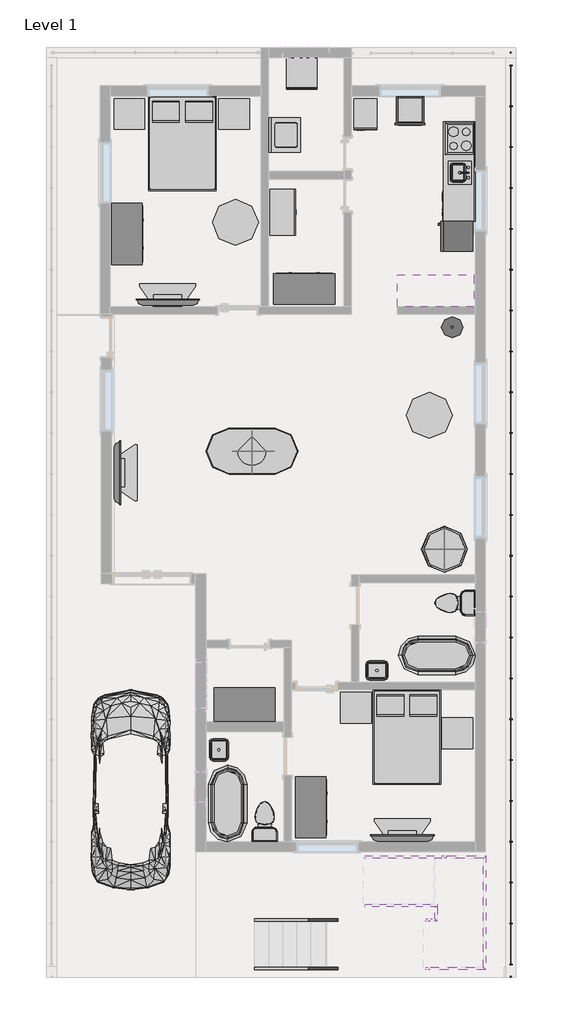
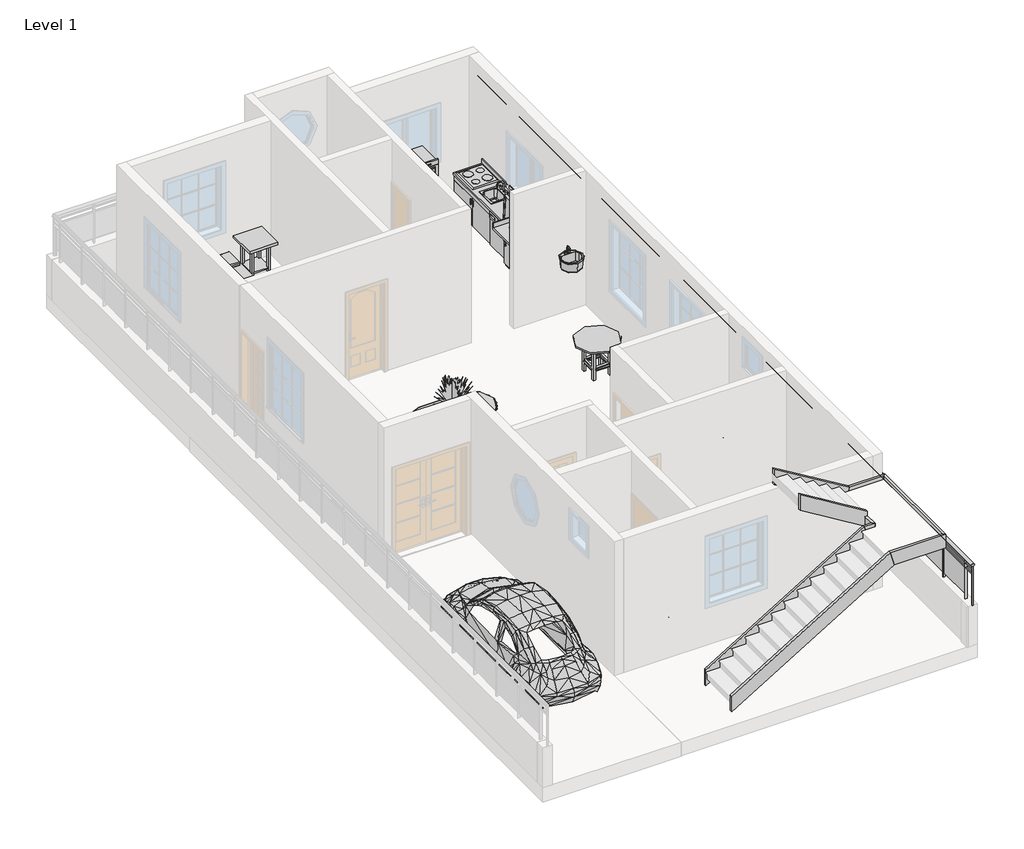
# One storey, part 3 of 3: 23 furniture elements, 9 members, 9 proxies, 8 flow terminals, 2 geographic elements, 1 railing.
"""IFC4 building model written with IfcOpenShell, lengths in millimetres."""

from ifc_helpers import new_model, si_unit, point, frame, origin, place, context, project, spatial, polyline, ellipse_curve, trimmed, outline, extrude, faceted_brep, transform, mapped, element, save
from ifc_brep_helpers import plane_surface, extruded_surface, advanced_brep
from components import proxy_7e1014cc, proxy_a6faaae8, proxy_45b28599, kitchenette_medium_kitchenette_medium_844211aa, proxy_8b8c2dc4, rpc_beetle_rpc_beetle_3ce7ba48, proxy_c523a7b7, proxy_718fa39f, flow_terminal_871c2e40, flow_terminal_d49f872f, flow_terminal_62a433f7, toilet_domestic_3d_toilet_domestic_3d_f7549cf7, toilet_domestic_3d_toilet_domestic_3d_183bbd19, flow_terminal_b374fae2, furniture_c8abb964, furniture_c6510c7c, furniture_6430aa70, furniture_2babcf72, furniture_9fa109b2, furniture_80f2079a, furniture_e1dba61b, furniture_fdf74506, tv_stand_tv_stand_6ce107e5, furniture_2c34a4f9, furniture_905aceb5, furniture_4bee3317, furniture_5bc9ed15, furniture_c80d6d9c, rpc_plant_tropical_agave_1_5_93a2a214, rpc_plant_tropical_dagger_2_80c14bd7

model = new_model("IFC4")

# Units and contexts
model_context = context("Model", 3, world=origin())
ifc_project = project(units=[si_unit("LENGTHUNIT", "METRE", prefix="MILLI")], contexts=[model_context])

# Site, building, storey
site = spatial("IfcSite", under=ifc_project)
building = spatial("IfcBuilding", under=site)
storey = spatial("IfcBuildingStorey", under=building, Name="Level 1", Elevation=0.0)

# Proxies
placement = place(None, origin())
proxy_shape = proxy_7e1014cc(model_context)
element("IfcBuildingElementProxy", 1, Name="18\" x 24\" x 34 1/2\"", ObjectType="18\" x 24\" x 34 1/2\"", at=placement, inside=storey, context=model_context, shape_type="MappedRepresentation", body=[
    mapped(proxy_shape, transform((-1733.5258635, 13886.7655534, 0.0), x_axis=(1.0, 0.0, 0.0), y_axis=(0.0, 1.0, 0.0), z_axis=(0.0, 0.0, 1.0))),
])
proxy_2_shape = proxy_a6faaae8(model_context)
element("IfcBuildingElementProxy", 2, Name="Cook Top-4 Unit2 : 22\" x 20\"", ObjectType="Cook Top-4 Unit2 : 22\" x 20\"", at=placement, inside=storey, context=model_context, shape_type="MappedRepresentation", body=[
    mapped(proxy_2_shape, transform((452.191605, 13657.9151182, 0.0), x_axis=(0.0, -1.0000000000000004, 0.0), y_axis=(1.0000000000000004, 0.0, 0.0), z_axis=(0.0, 0.0, 1.0))),
])
proxy_3_shape = proxy_45b28599(model_context)
element("IfcBuildingElementProxy", 3, Name="Dishwasher : 24\" x 24\" x 34\"", ObjectType="Dishwasher : 24\" x 24\" x 34\"", at=placement, inside=storey, context=model_context, shape_type="MappedRepresentation", body=[
    mapped(proxy_3_shape, transform((-3079.7258635, 14699.5655534, 0.0), x_axis=(1.0, 0.0, 0.0), y_axis=(0.0, 1.0, 0.0), z_axis=(0.0, 0.0, 1.0))),
])
element("IfcBuildingElementProxy", 4, Name="Dishwasher : 24\" x 24\" x 34\"", ObjectType="Dishwasher : 24\" x 24\" x 34\"", at=placement, inside=storey, context=model_context, shape_type="MappedRepresentation", body=[
    mapped(proxy_3_shape, transform((160.3420402, 12706.7325867, 0.0), x_axis=(0.0, -1.0000000000000004, 0.0), y_axis=(1.0000000000000004, 0.0, 0.0), z_axis=(0.0, 0.0, 1.0))),
])
kitchenette_medium_kitchenette_medium_shape = kitchenette_medium_kitchenette_medium_844211aa(model_context)
element("IfcBuildingElementProxy", 5, Name="Kitchenette - Medium : Kitchenette - Medium", ObjectType="Kitchenette - Medium : Kitchenette - Medium", at=placement, inside=storey, context=model_context, shape_type="MappedRepresentation", body=[
    mapped(kitchenette_medium_kitchenette_medium_shape, transform((756.991605, 13333.7528231, 0.0), x_axis=(0.0, -1.0000000000000004, 0.0), y_axis=(1.0000000000000004, 0.0, 0.0), z_axis=(0.0, 0.0, 1.0))),
])
proxy_4_shape = proxy_8b8c2dc4(model_context)
element("IfcBuildingElementProxy", 6, Name="Oven Double-Built-in : 21 1/2\" x 39 1/4\" x 21\"", ObjectType="Oven Double-Built-in : 21 1/2\" x 39 1/4\" x 21\"", at=placement, inside=storey, context=model_context, shape_type="MappedRepresentation", body=[
    mapped(proxy_4_shape, transform((-503.2334677, 14088.3492592, 0.0), x_axis=(1.0, 0.0, 0.0), y_axis=(0.0, 1.0, 0.0), z_axis=(0.0, 0.0, 1.0))),
])
rpc_beetle_rpc_beetle_shape = rpc_beetle_rpc_beetle_3ce7ba48(model_context)
element("IfcBuildingElementProxy", 7, Name="RPC Beetle : RPC Beetle", ObjectType="RPC Beetle : RPC Beetle", at=placement, inside=storey, context=model_context, shape_type="MappedRepresentation", body=[
    mapped(rpc_beetle_rpc_beetle_shape, transform((-6101.008395, -527.9848818, 0.0), x_axis=(1.0, 0.0, 0.0), y_axis=(0.0, 1.0, 0.0), z_axis=(0.0, 0.0, 1.0))),
])
proxy_5_shape = proxy_c523a7b7(model_context)
element("IfcBuildingElementProxy", 8, Name="Refrigerator : 24\" x 25\" LH", ObjectType="Refrigerator : 24\" x 25\" LH", at=placement, inside=storey, context=model_context, shape_type="MappedRepresentation", body=[
    mapped(proxy_5_shape, transform((406.5426335, 11721.1651182, 0.0), x_axis=(0.0, -1.0000000000000004, 0.0), y_axis=(1.0000000000000004, 0.0, 0.0), z_axis=(0.0, 0.0, 1.0))),
])
proxy_6_shape = proxy_718fa39f(model_context)
element("IfcBuildingElementProxy", 9, Name="Washer : 27\" x 25\" x 35\"", ObjectType="Washer : 27\" x 25\" x 35\"", at=placement, inside=storey, context=model_context, shape_type="MappedRepresentation", body=[
    mapped(proxy_6_shape, transform((-2761.1588302, 13313.6976497, 0.0), x_axis=(0.0, 1.0000000000000002, 0.0), y_axis=(-1.0000000000000002, 0.0, 0.0), z_axis=(0.0, 0.0, 1.0))),
])

# Flow terminals
flow_terminal_shape = flow_terminal_871c2e40(model_context)
element("IfcFlowTerminal", 10, ObjectType="Sink Kitchen-Island : 18\" x 18\"", at=placement, inside=storey, context=model_context, shape_type="MappedRepresentation", body=[
    mapped(flow_terminal_shape, transform((449.8462039, 13000.5043587, -14.4), x_axis=(0.0, -1.0000000000000004, 0.0), y_axis=(1.0000000000000004, 0.0, 0.0), z_axis=(0.0, 0.0, 1.0))),
])
flow_terminal_2_shape = flow_terminal_d49f872f(model_context)
element("IfcFlowTerminal", 11, ObjectType="Sink Vanity-Round : 19\" x 19\"", at=placement, inside=storey, context=model_context, shape_type="MappedRepresentation", body=[
    mapped(flow_terminal_2_shape, transform((203.1398644, 9824.9372099, 609.6), x_axis=(1.0, 0.0, 0.0), y_axis=(0.0, 1.0, 0.0), z_axis=(0.0, 0.0, 1.0))),
])
flow_terminal_3_shape = flow_terminal_62a433f7(model_context)
element("IfcFlowTerminal", 12, ObjectType="Sink Vanity-Square : 20\" x 18\"", at=placement, inside=storey, context=model_context, shape_type="MappedRepresentation", body=[
    mapped(flow_terminal_3_shape, transform((-4396.8629939, 1488.3258776, 609.6), x_axis=(0.0, 1.0, 0.0), y_axis=(-1.0, 0.0, 0.0), z_axis=(0.0, 0.0, 1.0))),
])
element("IfcFlowTerminal", 13, ObjectType="Sink Vanity-Square : 20\" x 18\"", at=placement, inside=storey, context=model_context, shape_type="MappedRepresentation", body=[
    mapped(flow_terminal_3_shape, transform((-1183.1191545, 3030.3605193, 609.6), x_axis=(-1.0000000000000002, 0.0, 0.0), y_axis=(0.0, -1.0000000000000002, 0.0), z_axis=(0.0, 0.0, 1.0))),
])
toilet_domestic_3d_toilet_domestic_3d_shape = toilet_domestic_3d_toilet_domestic_3d_f7549cf7(model_context)
toilet_domestic_3d_toilet_domestic_3d_2_shape = toilet_domestic_3d_toilet_domestic_3d_183bbd19(model_context)
element("IfcFlowTerminal", 14, ObjectType="Toilet-Domestic-3D : Toilet-Domestic-3D", at=placement, inside=storey, context=model_context, shape_type="MappedRepresentation", body=[
    mapped(toilet_domestic_3d_toilet_domestic_3d_shape, transform((262.2955776, 4425.0151182, 0.0), x_axis=(0.0, -1.0000000000000004, 0.0), y_axis=(1.0000000000000004, 0.0, 0.0), z_axis=(0.0, 0.0, 1.0))),
    mapped(toilet_domestic_3d_toilet_domestic_3d_2_shape, transform((262.2955776, 4425.0151182, 0.0), x_axis=(0.0, -1.0000000000000004, 0.0), y_axis=(1.0000000000000004, 0.0, 0.0), z_axis=(0.0, 0.0, 1.0))),
])
element("IfcFlowTerminal", 15, ObjectType="Toilet-Domestic-3D : Toilet-Domestic-3D", at=placement, inside=storey, context=model_context, shape_type="MappedRepresentation", body=[
    mapped(toilet_domestic_3d_toilet_domestic_3d_shape, transform((-3434.008395, 169.9111455, 0.0), x_axis=(-1.0000000000000004, 0.0, 0.0), y_axis=(0.0, -1.0000000000000004, 0.0), z_axis=(0.0, 0.0, 1.0))),
    mapped(toilet_domestic_3d_toilet_domestic_3d_2_shape, transform((-3434.008395, 169.9111455, 0.0), x_axis=(-1.0000000000000004, 0.0, 0.0), y_axis=(0.0, -1.0000000000000004, 0.0), z_axis=(0.0, 0.0, 1.0))),
])
flow_terminal_4_shape = flow_terminal_b374fae2(model_context)
element("IfcFlowTerminal", 16, ObjectType="Tub-Free Standing-3D : 30\" x 60\"", at=placement, inside=storey, context=model_context, shape_type="MappedRepresentation", body=[
    mapped(flow_terminal_4_shape, transform((-4170.608395, 437.2151182, 0.0), x_axis=(-1.0000000000000009, 0.0, 0.0), y_axis=(0.0, -1.0000000000000009, 0.0), z_axis=(0.0, 0.0, 1.0))),
])
element("IfcFlowTerminal", 17, ObjectType="Tub-Free Standing-3D : 30\" x 60\"", at=placement, inside=storey, context=model_context, shape_type="MappedRepresentation", body=[
    mapped(flow_terminal_4_shape, transform((-5.008395, 3383.6151182, 0.0), x_axis=(0.0, -1.0, 0.0), y_axis=(1.0, 0.0, 0.0), z_axis=(0.0, 0.0, 1.0))),
])

# Furniture
furniture_shape = furniture_c8abb964(model_context)
element("IfcFurniture", 18, ObjectType="Bed-Box : Double 53\" x 74\"", at=placement, inside=storey, context=model_context, shape_type="MappedRepresentation", body=[
    mapped(furniture_shape, transform((-941.0608541, 1992.4446264, 0.0), x_axis=(1.0, 0.0, 0.0), y_axis=(0.0, 1.0, 0.0), z_axis=(0.0, 0.0, 1.0))),
])
element("IfcFurniture", 19, ObjectType="Bed-Box : Double 53\" x 74\"", at=placement, inside=storey, context=model_context, shape_type="MappedRepresentation", body=[
    mapped(furniture_shape, transform((-5411.4608541, 13803.4446264, 0.0), x_axis=(1.0, 0.0, 0.0), y_axis=(0.0, 1.0, 0.0), z_axis=(0.0, 0.0, 1.0))),
])
furniture_2_shape = furniture_c6510c7c(model_context)
element("IfcFurniture", 20, ObjectType="Counter Top w Sink Hole : 24\" Depth", at=placement, inside=storey, context=model_context, shape_type="MappedRepresentation", body=[
    mapped(furniture_2_shape, transform((756.991605, 12800.3528231, -14.4), x_axis=(0.0, -1.0000000000000004, 0.0), y_axis=(1.0000000000000004, 0.0, 0.0), z_axis=(0.0, 0.0, 1.0))),
])
furniture_3_shape = furniture_6430aa70(model_context)
element("IfcFurniture", 21, ObjectType="Counter Top w Sink Hole : 24\" Depth", at=placement, inside=storey, context=model_context, shape_type="MappedRepresentation", body=[
    mapped(furniture_3_shape, transform((408.0539, 10952.8151182, 914.4), x_axis=(1.0, 0.0, 0.0), y_axis=(0.0, 1.0, 0.0), z_axis=(0.0, 0.0, 1.0))),
])
furniture_4_shape = furniture_2babcf72(model_context)
element("IfcFurniture", 22, ObjectType="Dresser : 48\" x 60\" x 24\"", at=placement, inside=storey, context=model_context, shape_type="MappedRepresentation", body=[
    mapped(furniture_4_shape, transform((-2915.8016549, 10310.2521641, 0.0), x_axis=(-1.0000000000000004, 0.0, 0.0), y_axis=(0.0, -1.0000000000000004, 0.0), z_axis=(0.0, 0.0, 1.0))),
])
furniture_5_shape = furniture_9fa109b2(model_context)
element("IfcFurniture", 23, ObjectType="Dresser : 48\" x 72\" x 24\"", at=placement, inside=storey, context=model_context, shape_type="MappedRepresentation", body=[
    mapped(furniture_5_shape, transform((-6540.3713491, 12034.808378, 0.0), x_axis=(0.0, 1.0000000000000009, 0.0), y_axis=(-1.0000000000000009, 0.0, 0.0), z_axis=(0.0, 0.0, 1.0))),
])
element("IfcFurniture", 24, ObjectType="Dresser : 48\" x 72\" x 24\"", at=placement, inside=storey, context=model_context, shape_type="MappedRepresentation", body=[
    mapped(furniture_5_shape, transform((-2882.7713491, 630.208378, 0.0), x_axis=(0.0, 1.0, 0.0), y_axis=(-1.0, 0.0, 0.0), z_axis=(0.0, 0.0, 1.0))),
])
furniture_6_shape = furniture_80f2079a(model_context)
element("IfcFurniture", 25, ObjectType="Entertainment Center : 72\" x 72\" x 24\"", at=placement, inside=storey, context=model_context, shape_type="MappedRepresentation", body=[
    mapped(furniture_6_shape, transform((-3833.8923341, 1961.2151182, 0.0), x_axis=(-1.0000000000000004, 0.0, 0.0), y_axis=(0.0, -1.0000000000000004, 0.0), z_axis=(0.0, 0.0, 1.0))),
])
furniture_7_shape = furniture_e1dba61b(model_context)
element("IfcFurniture", 26, ObjectType="Storage Pedestal : 20\" x 36\" x 36\"", at=placement, inside=storey, context=model_context, shape_type="MappedRepresentation", body=[
    mapped(furniture_7_shape, transform((-4012.7267711, 12377.4376321, 0.0), x_axis=(0.0, 1.000000000000001, 0.0), y_axis=(-1.000000000000001, 0.0, 0.0), z_axis=(0.0, 0.0, 1.0))),
])
furniture_8_shape = furniture_fdf74506(model_context)
element("IfcFurniture", 27, ObjectType="TV - Flat Screen : 50\"", at=placement, inside=storey, context=model_context, shape_type="MappedRepresentation", body=[
    mapped(furniture_8_shape, transform((-5368.3529092, 10401.7537418, 914.4), x_axis=(-1.0, 0.0, 0.0), y_axis=(0.0, -1.0, 0.0), z_axis=(0.0, 0.0, 1.0))),
])
element("IfcFurniture", 28, ObjectType="TV - Flat Screen : 50\"", at=placement, inside=storey, context=model_context, shape_type="MappedRepresentation", body=[
    mapped(furniture_8_shape, transform((-694.7529092, -253.5462582, 914.4), x_axis=(-1.0, 0.0, 0.0), y_axis=(0.0, -1.0, 0.0), z_axis=(0.0, 0.0, 1.0))),
])
element("IfcFurniture", 29, ObjectType="TV - Flat Screen : 50\"", at=placement, inside=storey, context=model_context, shape_type="MappedRepresentation", body=[
    mapped(furniture_8_shape, transform((-6372.6697714, 7019.7596323, 914.4), x_axis=(0.0, 1.0000000000000002, 0.0), y_axis=(-1.0000000000000002, 0.0, 0.0), z_axis=(0.0, 0.0, 1.0))),
])
tv_stand_tv_stand_shape = tv_stand_tv_stand_6ce107e5(model_context)
element("IfcFurniture", 30, ObjectType="TV Stand : TV Stand", at=placement, inside=storey, context=model_context, shape_type="MappedRepresentation", body=[
    mapped(tv_stand_tv_stand_shape, transform((-565.620393, -324.7848818, 0.0), x_axis=(-1.0000000000000007, 0.0, 0.0), y_axis=(0.0, -1.0000000000000007, 0.0), z_axis=(0.0, 0.0, 1.0))),
])
element("IfcFurniture", 31, ObjectType="TV Stand : TV Stand", at=placement, inside=storey, context=model_context, shape_type="MappedRepresentation", body=[
    mapped(tv_stand_tv_stand_shape, transform((-5239.220393, 10317.8151182, 0.0), x_axis=(-1.0, 0.0, 0.0), y_axis=(0.0, -1.0, 0.0), z_axis=(0.0, 0.0, 1.0))),
])
element("IfcFurniture", 32, ObjectType="TV Stand : TV Stand", at=placement, inside=storey, context=model_context, shape_type="MappedRepresentation", body=[
    mapped(tv_stand_tv_stand_shape, transform((-6431.208395, 6890.6271161, 0.0), x_axis=(0.0, 1.0000000000000002, 0.0), y_axis=(-1.0000000000000002, 0.0, 0.0), z_axis=(0.0, 0.0, 1.0))),
])
furniture_9_shape = furniture_2c34a4f9(model_context)
element("IfcFurniture", 33, ObjectType="Table-Dining Oval : 36\" x 72\"", at=placement, inside=storey, context=model_context, shape_type="MappedRepresentation", body=[
    mapped(furniture_9_shape, transform((-3286.1887229, 7805.7134788, 0.0), x_axis=(1.0, 0.0, 0.0), y_axis=(0.0, 1.0, 0.0), z_axis=(0.0, 0.0, 1.0))),
])
furniture_10_shape = furniture_905aceb5(model_context)
element("IfcFurniture", 34, ObjectType="Table-Dining Round w Chairs : 36\" Diameter", at=placement, inside=storey, context=model_context, shape_type="MappedRepresentation", body=[
    mapped(furniture_10_shape, transform((-261.0903622, 8343.6938067, 0.0), x_axis=(1.0, 0.0, 0.0), y_axis=(0.0, 1.0, 0.0), z_axis=(0.0, 0.0, 1.0))),
])
furniture_11_shape = furniture_4bee3317(model_context)
element("IfcFurniture", 35, ObjectType="Table-Ellipse : 72\" x 36\"", at=placement, inside=storey, context=model_context, shape_type="MappedRepresentation", body=[
    mapped(furniture_11_shape, transform((-4018.208395, 11994.2151182, 0.0), x_axis=(0.0, 1.0000000000000002, 0.0), y_axis=(-1.0000000000000002, 0.0, 0.0), z_axis=(0.0, 0.0, 1.0))),
])
furniture_12_shape = furniture_5bc9ed15(model_context)
element("IfcFurniture", 36, ObjectType="Table-Night Stand : 24\" x 24\" x 30\"", at=placement, inside=storey, context=model_context, shape_type="MappedRepresentation", body=[
    mapped(furniture_12_shape, transform((-6434.9420253, 13848.4151182, 0.0), x_axis=(1.0, 0.0, 0.0), y_axis=(0.0, 1.0, 0.0), z_axis=(0.0, 0.0, 1.0))),
])
element("IfcFurniture", 37, ObjectType="Table-Night Stand : 24\" x 24\" x 30\"", at=placement, inside=storey, context=model_context, shape_type="MappedRepresentation", body=[
    mapped(furniture_12_shape, transform((-4352.1420253, 13848.4151182, 0.0), x_axis=(1.0, 0.0, 0.0), y_axis=(0.0, 1.0, 0.0), z_axis=(0.0, 0.0, 1.0))),
])
element("IfcFurniture", 38, ObjectType="Table-Night Stand : 24\" x 24\" x 30\"", at=placement, inside=storey, context=model_context, shape_type="MappedRepresentation", body=[
    mapped(furniture_12_shape, transform((-1926.4420253, 2037.4151182, 0.0), x_axis=(1.0, 0.0, 0.0), y_axis=(0.0, 1.0, 0.0), z_axis=(0.0, 0.0, 1.0))),
])
element("IfcFurniture", 39, ObjectType="Table-Night Stand : 24\" x 24\" x 30\"", at=placement, inside=storey, context=model_context, shape_type="MappedRepresentation", body=[
    mapped(furniture_12_shape, transform((92.8579747, 1529.4151182, 0.0), x_axis=(1.0, 0.0, 0.0), y_axis=(0.0, 1.0, 0.0), z_axis=(0.0, 0.0, 1.0))),
])
furniture_13_shape = furniture_c80d6d9c(model_context)
element("IfcFurniture", 40, ObjectType="Table-Round : 36\" Diameter", at=placement, inside=storey, context=model_context, shape_type="MappedRepresentation", body=[
    mapped(furniture_13_shape, transform((147.391605, 5491.8151182, 0.0), x_axis=(1.0, 0.0, 0.0), y_axis=(0.0, 1.0, 0.0), z_axis=(0.0, 0.0, 1.0))),
])

# Geographic elements
rpc_plant_tropical_agave_1_5_shape = rpc_plant_tropical_agave_1_5_93a2a214(model_context)
element("IfcGeographicElement", 41, ObjectType="RPC Plant - Tropical : Agave - 1.5'", at=placement, inside=storey, context=model_context, shape_type="MappedRepresentation", body=[
    mapped(rpc_plant_tropical_agave_1_5_shape, transform((147.391605, 5491.8151182, 762.0), x_axis=(1.0, 0.0, 0.0), y_axis=(0.0, 1.0, 0.0), z_axis=(0.0, 0.0, 1.0))),
])
rpc_plant_tropical_dagger_2_shape = rpc_plant_tropical_dagger_2_80c14bd7(model_context)
element("IfcGeographicElement", 42, ObjectType="RPC Plant - Tropical : Dagger - 2'", at=placement, inside=storey, context=model_context, shape_type="MappedRepresentation", body=[
    mapped(rpc_plant_tropical_dagger_2_shape, transform((-3688.008395, 7447.6151182, 914.4), x_axis=(1.0, 0.0, 0.0), y_axis=(0.0, 1.0, 0.0), z_axis=(0.0, 0.0, 1.0))),
])

# Members
element("IfcMember", 43, ObjectType="Stringer - 2\" Width", at=placement, inside=storey, context=model_context, shape_type="SweptSolid", body=[
    extrude(outline(polyline([(550.7811786, -3631.685793), (194.3724171, -3631.685793), (2311.4, -138.5902812), (2616.2, -223.7447377), (550.7811786, -3631.685793)])), frame((0.0, -1908.8158798, 0.0), z_axis=(0.0, 1.0, 0.0), x_axis=(0.0, 0.0, 1.0)), (0.0, 0.0, 1.0), 50.8),
])
element("IfcMember", 44, ObjectType="Stringer - 2\" Width", at=placement, inside=storey, context=model_context, shape_type="SweptSolid", body=[
    extrude(outline(polyline([(550.7811786, -3631.685793), (194.3724171, -3631.685793), (2311.4, -138.5902812), (2616.2, -223.7447377), (550.7811786, -3631.685793)])), frame((0.0, -2874.0158798, 0.0), z_axis=(0.0, 1.0, 0.0), x_axis=(0.0, 0.0, 1.0)), (0.0, 0.0, 1.0), 50.8),
])
element("IfcMember", 45, ObjectType="Stringer - 2\" Width", at=placement, inside=storey, context=model_context, shape_type="SweptSolid", body=[
    extrude(outline(polyline([(2364.9178717, 7.691605), (2721.3266332, 7.691605), (3598.7811786, -1440.108395), (3242.3724171, -1440.108395), (2364.9178717, 7.691605)])), frame((0.0, -1620.1848818, 0.0), z_axis=(0.0, 1.0, 0.0), x_axis=(0.0, 0.0, 1.0)), (0.0, 0.0, 1.0), 50.8),
])
element("IfcMember", 46, ObjectType="Stringer - 2\" Width", at=placement, inside=storey, context=model_context, shape_type="SweptSolid", body=[
    extrude(outline(polyline([(2311.4, 95.9960932), (2616.2, 181.1505497), (3598.7811786, -1440.108395), (3242.3724171, -1440.108395), (2311.4, 95.9960932)])), frame((0.0, -654.9848818, 0.0), z_axis=(0.0, 1.0, 0.0), x_axis=(0.0, 0.0, 1.0)), (0.0, 0.0, 1.0), 50.8),
])
element("IfcMember", 47, ObjectType="Stringer - 2\" Width", at=placement, inside=storey, context=model_context, shape_type="SweptSolid", body=[
    extrude(outline(polyline([(-43.108395, -1620.1848818), (7.691605, -1620.1848818), (7.691605, -1908.8158798), (-43.108395, -1858.0158798), (-43.108395, -1620.1848818)])), frame((0.0, 0.0, 2311.4), z_axis=(0.0, 0.0, 1.0), x_axis=(1.0, 0.0, 0.0)), (0.0, 0.0, 1.0), 304.8),
])
element("IfcMember", 48, ObjectType="Stringer - 2\" Width", at=placement, inside=storey, context=model_context, shape_type="Brep", body=[
    faceted_brep([(-223.7447377, -2823.2158798, 2616.2), (-223.7447377, -2874.0158798, 2616.2), (972.891605, -2874.0158798, 2616.2), (922.091605, -2823.2158798, 2616.2), (-138.5902812, -2823.2158798, 2311.4), (922.091605, -2823.2158798, 2311.4), (-138.5902812, -2874.0158798, 2311.4), (972.891605, -2874.0158798, 2311.4)], [[[0, 1, 2, 3]], [[4, 0, 3, 5]], [[6, 4, 5, 7]], [[1, 6, 7, 2]], [[1, 0, 4, 6]], [[2, 7, 5, 3]]]),
])
element("IfcMember", 49, ObjectType="Stringer - 2\" Width", at=placement, inside=storey, context=model_context, shape_type="SweptSolid", body=[
    extrude(outline(polyline([(972.891605, -2874.0158798), (922.091605, -2823.2158798), (922.091605, -654.9848818), (972.891605, -604.1848818), (972.891605, -2874.0158798)])), frame((0.0, 0.0, 2311.4), z_axis=(0.0, 0.0, 1.0), x_axis=(1.0, 0.0, 0.0)), (0.0, 0.0, 1.0), 304.8),
])
element("IfcMember", 50, ObjectType="Stringer - 2\" Width", at=placement, inside=storey, context=model_context, shape_type="Brep", body=[
    faceted_brep([(7.691605, -1908.8158798, 2616.2), (-43.108395, -1858.0158798, 2616.2), (-223.7447377, -1858.0158798, 2616.2), (-223.7447377, -1908.8158798, 2616.2), (7.691605, -1908.8158798, 2311.4), (-138.5902812, -1908.8158798, 2311.4), (-43.108395, -1858.0158798, 2311.4), (-138.5902812, -1858.0158798, 2311.4)], [[[0, 1, 2, 3]], [[4, 0, 3, 5]], [[6, 4, 5, 7]], [[1, 6, 7, 2]], [[1, 0, 4, 6]], [[2, 7, 5, 3]]]),
])
element("IfcMember", 51, ObjectType="Stringer - 2\" Width", at=placement, inside=storey, context=model_context, shape_type="Brep", body=[
    faceted_brep([(922.091605, -654.9848818, 2616.2), (972.891605, -604.1848818, 2616.2), (181.1505497, -604.1848818, 2616.2), (181.1505497, -654.9848818, 2616.2), (922.091605, -654.9848818, 2311.4), (95.9960932, -654.9848818, 2311.4), (972.891605, -604.1848818, 2311.4), (95.9960932, -604.1848818, 2311.4)], [[[0, 1, 2, 3]], [[4, 0, 3, 5]], [[6, 4, 5, 7]], [[1, 6, 7, 2]], [[1, 0, 4, 6]], [[2, 7, 5, 3]]]),
])

# Railing
element("IfcRailing", 52, ObjectType="Glass Panel - Bottom Fill", at=placement, inside=storey, context=model_context, shape_type="SolidModel", body=[
    advanced_brep(
    [(1430.091605, -3017.1848818, 1828.8), (1506.291605, -3017.1848818, 1828.8), (1430.091605, 15372.4151182, 1828.8), (1506.291605, 15372.4151182, 1828.8)],
    [
        (0, 1, ellipse_curve(frame((1468.191605, -3017.1848818, 1828.8), z_axis=(0.0, -1.0, 0.0), x_axis=(1.0, 0.0, 0.0)), 38.1, 28.575)),
        (1, 0, ellipse_curve(frame((1468.191605, -3017.1848818, 1828.8), z_axis=(0.0, -1.0, 0.0), x_axis=(1.0, 0.0, 0.0)), 38.1, 28.575)),
        (2, 3, ellipse_curve(frame((1468.191605, 15372.4151182, 1828.8), z_axis=(0.0, 1.0, 0.0), x_axis=(1.0, 0.0, 0.0)), 38.1, 28.575)),
        (3, 2, ellipse_curve(frame((1468.191605, 15372.4151182, 1828.8), z_axis=(0.0, 1.0, 0.0), x_axis=(1.0, 0.0, 0.0)), 38.1, 28.575)),
        (0, 2),
        (3, 1),
    ],
    [
        plane_surface(frame((1468.191605, -3017.1848818, 1828.8), z_axis=(0.0, -1.0, 0.0), x_axis=(0.0, 0.0, 1.0))),
        plane_surface(frame((1468.191605, 15372.4151182, 1828.8), z_axis=(0.0, 1.0, 0.0), x_axis=(0.0, 0.0, 1.0))),
        extruded_surface(trimmed(ellipse_curve(frame((1468.191605, 15372.4151182, 1828.8), z_axis=(0.0, -1.0, 0.0), x_axis=(1.0, 0.0, 0.0)), 38.1, 28.575), [point((1430.091605, 15372.4151182, 1828.8))], [point((1506.291605, 15372.4151182, 1828.8))], True, "CARTESIAN"), (0.0, -18389.6, 0.0), 18389.6),
        extruded_surface(trimmed(ellipse_curve(frame((1468.191605, 15372.4151182, 1828.8), z_axis=(0.0, -1.0, 0.0), x_axis=(1.0, 0.0, 0.0)), 38.1, 28.575), [point((1506.291605, 15372.4151182, 1828.8))], [point((1430.091605, 15372.4151182, 1828.8))], True, "CARTESIAN"), (0.0, -18389.6, 0.0), 18389.6),
    ],
    [
        (0, [[1, 2]]),
        (1, [[3, 4]]),
        (2, [[-1, 5, -4, 6]]),
        (3, [[-2, -6, -3, -5]]),
    ],
),
    extrude(outline(polyline([(1480.891605, -3017.1848818), (1455.491605, -3017.1848818), (1455.491605, 15372.4151182), (1480.891605, 15372.4151182), (1480.891605, -3017.1848818)])), frame((0.0, 0.0, 1714.5), z_axis=(0.0, 0.0, 1.0), x_axis=(1.0, 0.0, 0.0)), (0.0, 0.0, 1.0), 25.4),
    extrude(outline(polyline([(1480.891605, -3017.1848818), (1455.491605, -3017.1848818), (1455.491605, 15372.4151182), (1480.891605, 15372.4151182), (1480.891605, -3017.1848818)])), frame((0.0, 0.0, 1612.9), z_axis=(0.0, 0.0, 1.0), x_axis=(1.0, 0.0, 0.0)), (0.0, 0.0, 1.0), 25.4),
    extrude(outline(polyline([(1493.591605, 15112.0651182), (1442.791605, 15112.0651182), (1442.791605, 15124.7651182), (1493.591605, 15124.7651182), (1493.591605, 15112.0651182)])), frame((0.0, 0.0, 914.4), z_axis=(0.0, 0.0, 1.0), x_axis=(1.0, 0.0, 0.0)), (0.0, 0.0, 1.0), 885.6788223),
    extrude(outline(polyline([(1461.656448, 14305.6151182), (1461.656448, 15118.4151182), (1468.006448, 15118.4151182), (1468.006448, 14305.6151182), (1461.656448, 14305.6151182)])), frame((0.0, 0.0, 1016.0), z_axis=(0.0, 0.0, 1.0), x_axis=(1.0, 0.0, 0.0)), (0.0, 0.0, 1.0), 596.9),
    extrude(outline(polyline([(1493.591605, 14299.2651182), (1442.791605, 14299.2651182), (1442.791605, 14311.9651182), (1493.591605, 14311.9651182), (1493.591605, 14299.2651182)])), frame((0.0, 0.0, 914.4), z_axis=(0.0, 0.0, 1.0), x_axis=(1.0, 0.0, 0.0)), (0.0, 0.0, 1.0), 885.6788223),
    extrude(outline(polyline([(1461.656448, 13492.8151182), (1461.656448, 14305.6151182), (1468.006448, 14305.6151182), (1468.006448, 13492.8151182), (1461.656448, 13492.8151182)])), frame((0.0, 0.0, 1016.0), z_axis=(0.0, 0.0, 1.0), x_axis=(1.0, 0.0, 0.0)), (0.0, 0.0, 1.0), 596.9),
    extrude(outline(polyline([(1493.591605, 13486.4651182), (1442.791605, 13486.4651182), (1442.791605, 13499.1651182), (1493.591605, 13499.1651182), (1493.591605, 13486.4651182)])), frame((0.0, 0.0, 914.4), z_axis=(0.0, 0.0, 1.0), x_axis=(1.0, 0.0, 0.0)), (0.0, 0.0, 1.0), 885.6788223),
    extrude(outline(polyline([(1461.656448, 12680.0151182), (1461.656448, 13492.8151182), (1468.006448, 13492.8151182), (1468.006448, 12680.0151182), (1461.656448, 12680.0151182)])), frame((0.0, 0.0, 1016.0), z_axis=(0.0, 0.0, 1.0), x_axis=(1.0, 0.0, 0.0)), (0.0, 0.0, 1.0), 596.9),
    extrude(outline(polyline([(1493.591605, 12673.6651182), (1442.791605, 12673.6651182), (1442.791605, 12686.3651182), (1493.591605, 12686.3651182), (1493.591605, 12673.6651182)])), frame((0.0, 0.0, 914.4), z_axis=(0.0, 0.0, 1.0), x_axis=(1.0, 0.0, 0.0)), (0.0, 0.0, 1.0), 885.6788223),
    extrude(outline(polyline([(1461.656448, 11867.2151182), (1461.656448, 12680.0151182), (1468.006448, 12680.0151182), (1468.006448, 11867.2151182), (1461.656448, 11867.2151182)])), frame((0.0, 0.0, 1016.0), z_axis=(0.0, 0.0, 1.0), x_axis=(1.0, 0.0, 0.0)), (0.0, 0.0, 1.0), 596.9),
    extrude(outline(polyline([(1493.591605, 11860.8651182), (1442.791605, 11860.8651182), (1442.791605, 11873.5651182), (1493.591605, 11873.5651182), (1493.591605, 11860.8651182)])), frame((0.0, 0.0, 914.4), z_axis=(0.0, 0.0, 1.0), x_axis=(1.0, 0.0, 0.0)), (0.0, 0.0, 1.0), 885.6788223),
    extrude(outline(polyline([(1461.656448, 11054.4151182), (1461.656448, 11867.2151182), (1468.006448, 11867.2151182), (1468.006448, 11054.4151182), (1461.656448, 11054.4151182)])), frame((0.0, 0.0, 1016.0), z_axis=(0.0, 0.0, 1.0), x_axis=(1.0, 0.0, 0.0)), (0.0, 0.0, 1.0), 596.9),
    extrude(outline(polyline([(1493.591605, 11048.0651182), (1442.791605, 11048.0651182), (1442.791605, 11060.7651182), (1493.591605, 11060.7651182), (1493.591605, 11048.0651182)])), frame((0.0, 0.0, 914.4), z_axis=(0.0, 0.0, 1.0), x_axis=(1.0, 0.0, 0.0)), (0.0, 0.0, 1.0), 885.6788223),
    extrude(outline(polyline([(1461.656448, 10241.6151182), (1461.656448, 11054.4151182), (1468.006448, 11054.4151182), (1468.006448, 10241.6151182), (1461.656448, 10241.6151182)])), frame((0.0, 0.0, 1016.0), z_axis=(0.0, 0.0, 1.0), x_axis=(1.0, 0.0, 0.0)), (0.0, 0.0, 1.0), 596.9),
    extrude(outline(polyline([(1493.591605, 10235.2651182), (1442.791605, 10235.2651182), (1442.791605, 10247.9651182), (1493.591605, 10247.9651182), (1493.591605, 10235.2651182)])), frame((0.0, 0.0, 914.4), z_axis=(0.0, 0.0, 1.0), x_axis=(1.0, 0.0, 0.0)), (0.0, 0.0, 1.0), 885.6788223),
    extrude(outline(polyline([(1461.656448, 9428.8151182), (1461.656448, 10241.6151182), (1468.006448, 10241.6151182), (1468.006448, 9428.8151182), (1461.656448, 9428.8151182)])), frame((0.0, 0.0, 1016.0), z_axis=(0.0, 0.0, 1.0), x_axis=(1.0, 0.0, 0.0)), (0.0, 0.0, 1.0), 596.9),
    extrude(outline(polyline([(1493.591605, 9422.4651182), (1442.791605, 9422.4651182), (1442.791605, 9435.1651182), (1493.591605, 9435.1651182), (1493.591605, 9422.4651182)])), frame((0.0, 0.0, 914.4), z_axis=(0.0, 0.0, 1.0), x_axis=(1.0, 0.0, 0.0)), (0.0, 0.0, 1.0), 885.6788223),
    extrude(outline(polyline([(1461.656448, 8616.0151182), (1461.656448, 9428.8151182), (1468.006448, 9428.8151182), (1468.006448, 8616.0151182), (1461.656448, 8616.0151182)])), frame((0.0, 0.0, 1016.0), z_axis=(0.0, 0.0, 1.0), x_axis=(1.0, 0.0, 0.0)), (0.0, 0.0, 1.0), 596.9),
    extrude(outline(polyline([(1493.591605, 8609.6651182), (1442.791605, 8609.6651182), (1442.791605, 8622.3651182), (1493.591605, 8622.3651182), (1493.591605, 8609.6651182)])), frame((0.0, 0.0, 914.4), z_axis=(0.0, 0.0, 1.0), x_axis=(1.0, 0.0, 0.0)), (0.0, 0.0, 1.0), 885.6788223),
    extrude(outline(polyline([(1461.656448, 7803.2151182), (1461.656448, 8616.0151182), (1468.006448, 8616.0151182), (1468.006448, 7803.2151182), (1461.656448, 7803.2151182)])), frame((0.0, 0.0, 1016.0), z_axis=(0.0, 0.0, 1.0), x_axis=(1.0, 0.0, 0.0)), (0.0, 0.0, 1.0), 596.9),
    extrude(outline(polyline([(1493.591605, 7796.8651182), (1442.791605, 7796.8651182), (1442.791605, 7809.5651182), (1493.591605, 7809.5651182), (1493.591605, 7796.8651182)])), frame((0.0, 0.0, 914.4), z_axis=(0.0, 0.0, 1.0), x_axis=(1.0, 0.0, 0.0)), (0.0, 0.0, 1.0), 885.6788223),
    extrude(outline(polyline([(1461.656448, 6990.4151182), (1461.656448, 7803.2151182), (1468.006448, 7803.2151182), (1468.006448, 6990.4151182), (1461.656448, 6990.4151182)])), frame((0.0, 0.0, 1016.0), z_axis=(0.0, 0.0, 1.0), x_axis=(1.0, 0.0, 0.0)), (0.0, 0.0, 1.0), 596.9),
    extrude(outline(polyline([(1493.591605, 6984.0651182), (1442.791605, 6984.0651182), (1442.791605, 6996.7651182), (1493.591605, 6996.7651182), (1493.591605, 6984.0651182)])), frame((0.0, 0.0, 914.4), z_axis=(0.0, 0.0, 1.0), x_axis=(1.0, 0.0, 0.0)), (0.0, 0.0, 1.0), 885.6788223),
    extrude(outline(polyline([(1461.656448, 6177.6151182), (1461.656448, 6990.4151182), (1468.006448, 6990.4151182), (1468.006448, 6177.6151182), (1461.656448, 6177.6151182)])), frame((0.0, 0.0, 1016.0), z_axis=(0.0, 0.0, 1.0), x_axis=(1.0, 0.0, 0.0)), (0.0, 0.0, 1.0), 596.9),
    extrude(outline(polyline([(1493.591605, 6171.2651182), (1442.791605, 6171.2651182), (1442.791605, 6183.9651182), (1493.591605, 6183.9651182), (1493.591605, 6171.2651182)])), frame((0.0, 0.0, 914.4), z_axis=(0.0, 0.0, 1.0), x_axis=(1.0, 0.0, 0.0)), (0.0, 0.0, 1.0), 885.6788223),
    extrude(outline(polyline([(1461.656448, 5364.8151182), (1461.656448, 6177.6151182), (1468.006448, 6177.6151182), (1468.006448, 5364.8151182), (1461.656448, 5364.8151182)])), frame((0.0, 0.0, 1016.0), z_axis=(0.0, 0.0, 1.0), x_axis=(1.0, 0.0, 0.0)), (0.0, 0.0, 1.0), 596.9),
    extrude(outline(polyline([(1493.591605, 5358.4651182), (1442.791605, 5358.4651182), (1442.791605, 5371.1651182), (1493.591605, 5371.1651182), (1493.591605, 5358.4651182)])), frame((0.0, 0.0, 914.4), z_axis=(0.0, 0.0, 1.0), x_axis=(1.0, 0.0, 0.0)), (0.0, 0.0, 1.0), 885.6788223),
    extrude(outline(polyline([(1461.656448, 4552.0151182), (1461.656448, 5364.8151182), (1468.006448, 5364.8151182), (1468.006448, 4552.0151182), (1461.656448, 4552.0151182)])), frame((0.0, 0.0, 1016.0), z_axis=(0.0, 0.0, 1.0), x_axis=(1.0, 0.0, 0.0)), (0.0, 0.0, 1.0), 596.9),
    extrude(outline(polyline([(1493.591605, 4545.6651182), (1442.791605, 4545.6651182), (1442.791605, 4558.3651182), (1493.591605, 4558.3651182), (1493.591605, 4545.6651182)])), frame((0.0, 0.0, 914.4), z_axis=(0.0, 0.0, 1.0), x_axis=(1.0, 0.0, 0.0)), (0.0, 0.0, 1.0), 885.6788223),
    extrude(outline(polyline([(1461.656448, 3739.2151182), (1461.656448, 4552.0151182), (1468.006448, 4552.0151182), (1468.006448, 3739.2151182), (1461.656448, 3739.2151182)])), frame((0.0, 0.0, 1016.0), z_axis=(0.0, 0.0, 1.0), x_axis=(1.0, 0.0, 0.0)), (0.0, 0.0, 1.0), 596.9),
    extrude(outline(polyline([(1493.591605, 3732.8651182), (1442.791605, 3732.8651182), (1442.791605, 3745.5651182), (1493.591605, 3745.5651182), (1493.591605, 3732.8651182)])), frame((0.0, 0.0, 914.4), z_axis=(0.0, 0.0, 1.0), x_axis=(1.0, 0.0, 0.0)), (0.0, 0.0, 1.0), 885.6788223),
    extrude(outline(polyline([(1461.656448, 2926.4151182), (1461.656448, 3739.2151182), (1468.006448, 3739.2151182), (1468.006448, 2926.4151182), (1461.656448, 2926.4151182)])), frame((0.0, 0.0, 1016.0), z_axis=(0.0, 0.0, 1.0), x_axis=(1.0, 0.0, 0.0)), (0.0, 0.0, 1.0), 596.9),
    extrude(outline(polyline([(1493.591605, 2920.0651182), (1442.791605, 2920.0651182), (1442.791605, 2932.7651182), (1493.591605, 2932.7651182), (1493.591605, 2920.0651182)])), frame((0.0, 0.0, 914.4), z_axis=(0.0, 0.0, 1.0), x_axis=(1.0, 0.0, 0.0)), (0.0, 0.0, 1.0), 885.6788223),
    extrude(outline(polyline([(1461.656448, 2113.6151182), (1461.656448, 2926.4151182), (1468.006448, 2926.4151182), (1468.006448, 2113.6151182), (1461.656448, 2113.6151182)])), frame((0.0, 0.0, 1016.0), z_axis=(0.0, 0.0, 1.0), x_axis=(1.0, 0.0, 0.0)), (0.0, 0.0, 1.0), 596.9),
    extrude(outline(polyline([(1493.591605, 2107.2651182), (1442.791605, 2107.2651182), (1442.791605, 2119.9651182), (1493.591605, 2119.9651182), (1493.591605, 2107.2651182)])), frame((0.0, 0.0, 914.4), z_axis=(0.0, 0.0, 1.0), x_axis=(1.0, 0.0, 0.0)), (0.0, 0.0, 1.0), 885.6788223),
    extrude(outline(polyline([(1461.656448, 1300.8151182), (1461.656448, 2113.6151182), (1468.006448, 2113.6151182), (1468.006448, 1300.8151182), (1461.656448, 1300.8151182)])), frame((0.0, 0.0, 1016.0), z_axis=(0.0, 0.0, 1.0), x_axis=(1.0, 0.0, 0.0)), (0.0, 0.0, 1.0), 596.9),
    extrude(outline(polyline([(1493.591605, 1294.4651182), (1442.791605, 1294.4651182), (1442.791605, 1307.1651182), (1493.591605, 1307.1651182), (1493.591605, 1294.4651182)])), frame((0.0, 0.0, 914.4), z_axis=(0.0, 0.0, 1.0), x_axis=(1.0, 0.0, 0.0)), (0.0, 0.0, 1.0), 885.6788223),
    extrude(outline(polyline([(1461.656448, 488.0151182), (1461.656448, 1300.8151182), (1468.006448, 1300.8151182), (1468.006448, 488.0151182), (1461.656448, 488.0151182)])), frame((0.0, 0.0, 1016.0), z_axis=(0.0, 0.0, 1.0), x_axis=(1.0, 0.0, 0.0)), (0.0, 0.0, 1.0), 596.9),
    extrude(outline(polyline([(1493.591605, 481.6651182), (1442.791605, 481.6651182), (1442.791605, 494.3651182), (1493.591605, 494.3651182), (1493.591605, 481.6651182)])), frame((0.0, 0.0, 914.4), z_axis=(0.0, 0.0, 1.0), x_axis=(1.0, 0.0, 0.0)), (0.0, 0.0, 1.0), 885.6788223),
    extrude(outline(polyline([(1461.656448, -324.7848818), (1461.656448, 488.0151182), (1468.006448, 488.0151182), (1468.006448, -324.7848818), (1461.656448, -324.7848818)])), frame((0.0, 0.0, 1016.0), z_axis=(0.0, 0.0, 1.0), x_axis=(1.0, 0.0, 0.0)), (0.0, 0.0, 1.0), 596.9),
    extrude(outline(polyline([(1493.591605, -331.1348818), (1442.791605, -331.1348818), (1442.791605, -318.4348818), (1493.591605, -318.4348818), (1493.591605, -331.1348818)])), frame((0.0, 0.0, 914.4), z_axis=(0.0, 0.0, 1.0), x_axis=(1.0, 0.0, 0.0)), (0.0, 0.0, 1.0), 885.6788223),
    extrude(outline(polyline([(1461.656448, -1137.5848818), (1461.656448, -324.7848818), (1468.006448, -324.7848818), (1468.006448, -1137.5848818), (1461.656448, -1137.5848818)])), frame((0.0, 0.0, 1016.0), z_axis=(0.0, 0.0, 1.0), x_axis=(1.0, 0.0, 0.0)), (0.0, 0.0, 1.0), 596.9),
    extrude(outline(polyline([(1493.591605, -1143.9348818), (1442.791605, -1143.9348818), (1442.791605, -1131.2348818), (1493.591605, -1131.2348818), (1493.591605, -1143.9348818)])), frame((0.0, 0.0, 914.4), z_axis=(0.0, 0.0, 1.0), x_axis=(1.0, 0.0, 0.0)), (0.0, 0.0, 1.0), 885.6788223),
    extrude(outline(polyline([(1461.656448, -1950.3848818), (1461.656448, -1137.5848818), (1468.006448, -1137.5848818), (1468.006448, -1950.3848818), (1461.656448, -1950.3848818)])), frame((0.0, 0.0, 1016.0), z_axis=(0.0, 0.0, 1.0), x_axis=(1.0, 0.0, 0.0)), (0.0, 0.0, 1.0), 596.9),
    extrude(outline(polyline([(1493.591605, -1956.7348818), (1442.791605, -1956.7348818), (1442.791605, -1944.0348818), (1493.591605, -1944.0348818), (1493.591605, -1956.7348818)])), frame((0.0, 0.0, 914.4), z_axis=(0.0, 0.0, 1.0), x_axis=(1.0, 0.0, 0.0)), (0.0, 0.0, 1.0), 885.6788223),
    extrude(outline(polyline([(1461.656448, -2763.1848818), (1461.656448, -1950.3848818), (1468.006448, -1950.3848818), (1468.006448, -2763.1848818), (1461.656448, -2763.1848818)])), frame((0.0, 0.0, 1016.0), z_axis=(0.0, 0.0, 1.0), x_axis=(1.0, 0.0, 0.0)), (0.0, 0.0, 1.0), 596.9),
    extrude(outline(polyline([(1493.591605, -2769.5348818), (1442.791605, -2769.5348818), (1442.791605, -2756.8348818), (1493.591605, -2756.8348818), (1493.591605, -2769.5348818)])), frame((0.0, 0.0, 914.4), z_axis=(0.0, 0.0, 1.0), x_axis=(1.0, 0.0, 0.0)), (0.0, 0.0, 1.0), 885.6788223),
    extrude(outline(polyline([(1477.716605, 15359.7151182), (1458.666605, 15359.7151182), (1458.666605, 15378.7651182), (1477.716605, 15378.7651182), (1477.716605, 15359.7151182)])), frame((0.0, 0.0, 914.4), z_axis=(0.0, 0.0, 1.0), x_axis=(1.0, 0.0, 0.0)), (0.0, 0.0, 1.0), 885.6788223),
    extrude(outline(polyline([(1477.716605, -3023.5348818), (1458.666605, -3023.5348818), (1458.666605, -3004.4848818), (1477.716605, -3004.4848818), (1477.716605, -3023.5348818)])), frame((0.0, 0.0, 914.4), z_axis=(0.0, 0.0, 1.0), x_axis=(1.0, 0.0, 0.0)), (0.0, 0.0, 1.0), 885.6788223),
])

save(model, "model.ifc")

# Revit data of these elements
# Type "18\" x 24\" x 34 1/2\""
#   Label = "T"
#   Assembly Code = "E1090400"
#   Depth = 2' - 0"
#   Height = 2' - 10 1/2"
#   Width = 1' - 6"
#   Panel Face Material = Plastic, Opaque Black
#   Trach Compact. Material = Steel, Paint Finish, Ivory, Matte
#   Default Elevation = 0
# Type "Cook Top-4 Unit2 : 22\" x 20\""
#   Depth = 1' - 8"
#   Width = 1' - 10"
#   Burner Material = Steel, Chrome Plated
#   Cooktop Material = Steel, Polished
#   Default Elevation = 0
#   Assembly Code = ""
# Type "Dishwasher : 24\" x 24\" x 34\""
#   Label = "DW"
#   Assembly Code = "E1090400"
#   Depth = 2' - 0"
#   Height = 2' - 10"
#   Width = 2' - 0"
#   Dishwasher Material = Steel, Paint Finish, Ivory, Glossy
#   Panel Face Material = Plastic, Opaque Black
#   Default Elevation = 0
# Type "Kitchenette - Medium : Kitchenette - Medium"
#   Assembly Code = "E1090400"
#   Counter Length = 6' - 6"
#   Cabinet Width = 4' - 6"
#   Cabinet Height = 2' - 10 1/2"
#   Cabinet Depth = 2' - 0"
#   Toe Depth = 0' - 3"
#   Toe Height = 0' - 3 1/2"
#   Cabinet Material = Cabinets
#   Door/Drawer Material = Cabinets
#   Handle Material = Cabinets - Handles
#   Default Elevation = 0
# Type "Oven Double-Built-in : 21 1/2\" x 39 1/4\" x 21\""
#   Label = "OVEN"
#   Assembly Code = "E1090400"
#   Depth = 1' - 9"
#   Height = 3' - 3 1/4"
#   Width = 1' - 9 1/2"
#   Oven Material = Metal - Stainless Steel, Polished
#   Default Elevation = 0
# Type "RPC Beetle : RPC Beetle"
#   built-in parameter 1005195 = "RPC-16-0U6E-L4EG-ENH1-J3KF-SVEL-0TX4-C0"
#   Height = 0
# Type "Refrigerator : 24\" x 25\" LH"
#   Label = "REF."
#   Assembly Code = "E1090400"
#   Depth = 2' - 0 3/4"
#   Handle = 0' - 1 1/2"
#   Height = 5' - 3 1/2"
#   Rear Clearance = 0' - 2"
#   Top Door Height = 1' - 8"
#   Width = 1' - 11 1/2"
#   Material = Steel, Paint Finish, Ivory, Glossy
#   Default Elevation = 0
# Type "Washer : 27\" x 25\" x 35\""
#   Label = "W"
#   Assembly Code = "E1090400"
#   Depth = 2' - 1"
#   Height = 2' - 11"
#   Width = 2' - 3"
#   Washer Material = Steel, Paint Finish, Ivory, Matte
#   Default Elevation = 0
# Type "Sink Kitchen-Island : 18\" x 18\""
#   Assembly Code = "D2010410"
#   Counter Height = 3' - 0"
#   Depth = 1' - 6"
#   Width = 1' - 6"
#   Faucet Material = Steel, Polished
#   Sink Material = Steel, Polished
#   Default Elevation = 0
# Type "Sink Vanity-Round : 19\" x 19\""
#   Assembly Code = "D2010400"
#   Top Of Counter = 2' - 7"
#   Basin Material = Porcelain, Linen
#   Faucet Material = Steel, Polished
#   Default Elevation = 0
# Type "Sink Vanity-Square : 20\" x 18\""
#   Assembly Code = "D2010400"
#   Counter Height = 2' - 7"
#   Depth = 1' - 6"
#   Width = 1' - 8"
#   Basin Material = Porcelain, Linen
#   Faucet Material = Steel, Polished
#   Default Elevation = 0
# Type "Toilet-Domestic-3D : Toilet-Domestic-3D"
#   Assembly Code = "D2010110"
#   Toilet - Bowl/Basin Material = Porcelain, Linen
#   Toilet - Seat Material = Laminate, Linen, Matte
#   Default Elevation = 0
# Type "Tub-Free Standing-3D : 30\" x 60\""
#   Assembly Code = "D2010110"
#   Height = 1' - 6"
#   Length = 5' - 0"
#   Width = 2' - 6"
#   Tub Material = Porcelain, Ivory
#   Default Elevation = 0
# Type "Bed-Box : Double 53\" x 74\""
#   Assembly Code = "E2020200"
#   Length = 6' - 2"
#   Width = 4' - 5"
#   Frame Material = Birch
#   Mattress Material = Linen, White
#   Default Elevation = 0
# Type "Counter Top w Sink Hole : 24\" Depth"
#   Assembly Code = "C1030400"
#   Counter Thickness = 0' - 1 1/2"
#   Depth = 2' - 1"
#   Height = 3' - 0"
#   Length [instance default] = 8' - 0"
#   Sink Location [instance default] = 2' - 0"
#   Sink Location To Wall [instance default] = 0' - 6"
#   Sink Opening Depth [instance default] = 1' - 3"
#   Sink Opening Width [instance default] = 2' - 3"
#   Counter Top Material = none
#   Default Elevation = 0
# Type "Dresser : 48\" x 60\" x 24\""
#   Assembly Code = "E2020200"
#   Depth = 2' - 0"
#   Height = 5' - 0"
#   Width = 4' - 0"
#   Dresser Material = Laminate - Ivory, Glossy
#   Drawer Material = Laminate, Ivory, Matte
#   Knob Material = Cherry
#   Default Elevation = 0
# Type "Dresser : 48\" x 72\" x 24\""
#   Assembly Code = "E2020200"
#   Depth = 2' - 0"
#   Height = 6' - 0"
#   Width = 4' - 0"
#   Dresser Material = Laminate - Ivory, Glossy
#   Drawer Material = Laminate, Ivory, Matte
#   Knob Material = Cherry
#   Default Elevation = 0
# Type "Entertainment Center : 72\" x 72\" x 24\""
#   Assembly Code = "E2020200"
#   Center Width = 2' - 8"
#   Depth = 2' - 0"
#   Height = 4' - 0"
#   Width = 4' - 0"
#   Material = none
#   Default Elevation = 0
# Type "Storage Pedestal : 20\" x 36\" x 36\""
#   Assembly Code = "E2020"
#   Depth = 1' - 8"
#   Height = 3' - 0"
#   Width = 3' - 0"
#   Cabinet Material = Steel, Paint Finish, Ivory, Glossy
#   Handles Material = Steel, Chrome Plated
#   Default Elevation = 0
# Type "TV - Flat Screen : 50\""
#   SinAng = 0' - 0.0193"
#   L = 3' - 7.57782"
#   H = 2' - 0.51477"
#   Thickness = 0' - 4.33071"
#   Diagonal = 4' - 2"
#   CosAng = 0' - 0.03431"
#   Stand [instance default] = yes
#   Default Elevation = 0
# Type "TV Stand : TV Stand"
#   Depth = 1' - 6"
#   Width = 3' - 8"
#   Height = 1' - 7 1/2"
#   Finish = Melamine - Gray
#   Default Elevation = 0
# Type "Table-Dining Oval : 36\" x 72\""
#   Assembly Code = "E2020200"
#   Length = 6' - 0"
#   Width = 3' - 0"
#   Base Material = Steel, Chrome Plated
#   Top Material = Glass - Clear, Grey
#   Default Elevation = 0
#   Description = (empty or 0)
# Type "Table-Dining Round w Chairs : 36\" Diameter"
#   Assembly Code = "E2020200"
#   Radius = 1' - 6"
#   Diameter = 3' - 0"
#   Height = 2' - 6"
#   Chairs = 4
#   Base Material = Pine
#   Top Material = Laminate, Linen, Matte
#   Default Elevation = 0
# Type "Table-Ellipse : 72\" x 36\""
#   Assembly Code = "E2020200"
#   Half Width = 1' - 6"
#   Half Length = 1' - 6"
#   Height = 2' - 6"
#   Length = 3' - 0"
#   Width = 3' - 0"
#   Base Material = Birch
#   Top Material = Laminate - Black
#   Default Elevation = 0
# Type "Table-Night Stand : 24\" x 24\" x 30\""
#   Assembly Code = "E2020200"
#   Depth = 2' - 0"
#   Height = 2' - 6"
#   Width = 2' - 0"
#   Base Material = Birch
#   Top Material = Laminate, Ivory, Matte
#   Default Elevation = 0
# Type "Table-Round : 36\" Diameter"
#   Assembly Code = "E2020200"
#   Base Radius = 0' - 10"
#   Height = 2' - 6"
#   Radius = 1' - 6"
#   Base Material = Steel, Chrome Plated
#   Top Material = Birch
#   Default Elevation = 0
# Type "RPC Plant - Tropical : Agave - 1.5'"
#   built-in parameter 1005198 = "{2, 15},{39, RPC-16-G1GJ-63FX-7K5P-N000-ST1L-LVER-AU},{1, 0},{1, 0},{2, 13},{1, 8},{5, Color},{1, 0},{1, 0},{3, 0.8},{3, 0.8},{3, 0.8},{1, 8},{7, BBoxMin},{1, 0},{1, 0},{1, 0},{1, 0},{1, 0},{1, 8},{7, BBoxMax},{1, 0},{1, 0},{1, 0},{1, 0},{1, 0},{2, 11},{9, RPCTypeId},{1, 0},{1, 0},{39, RPC-16-G1GJ-63FX-7K5P-N000-ST1L-LVER-AU},{1, 6},{14, RPCPlantHeight},{1, 0},{1, 0},{3, 1.5},{2, 11},{7, keyword},{1, 0},{1, 0},{35, :RPCs:Plants [General]:Geometry:RPC},{2, 11},{8, category},{1, 0},{1, 0},{16, Plants [General]},{2, 11},{12, LocalizedUID},{1, 0},{1, 0},{5, Agave},{2, 14},{6, Height},{1, 0},{1, 0},{3, 1.5},{1, 2},{16, Cast Reflections},{1, 0},{1, 0},{1, 0},{1, 2},{12, Cast Shadows},{1, 0},{1, 0},{1, 1},{1, 2},{9, Lock View},{1, 0},{1, 0},{1, 0},{1, 4},{5, ViewC},{1, 0},{1, 0},{1, 0},{21, assetlibrary_base.fbx},{1, 5},"
#   built-in parameter 1005195 = "RPC-16-G1GJ-63FX-7K5P-N000-ST1L-LVER-AU"
#   Type Comments = "Agave"
#   Assembly Code = "G2050500"
#   Height = 1' - 6"
#   Default Elevation = 0
# Type "RPC Plant - Tropical : Dagger - 2'"
#   built-in parameter 1005198 = "{2, 15},{39, RPC-16-G3A7-NEG0-UH6H-J000-ST1L-LVER-AU},{1, 0},{1, 0},{2, 13},{1, 8},{5, Color},{1, 0},{1, 0},{3, 0.8},{3, 0.8},{3, 0.8},{1, 8},{7, BBoxMin},{1, 0},{1, 0},{1, 0},{1, 0},{1, 0},{1, 8},{7, BBoxMax},{1, 0},{1, 0},{1, 0},{1, 0},{1, 0},{2, 11},{9, RPCTypeId},{1, 0},{1, 0},{39, RPC-16-G3A7-NEG0-UH6H-J000-ST1L-LVER-AU},{1, 6},{14, RPCPlantHeight},{1, 0},{1, 0},{1, 2},{2, 11},{7, keyword},{1, 0},{1, 0},{35, :RPCs:Plants [General]:Geometry:RPC},{2, 11},{8, category},{1, 0},{1, 0},{16, Plants [General]},{2, 11},{12, LocalizedUID},{1, 0},{1, 0},{6, Dagger},{2, 14},{6, Height},{1, 0},{1, 0},{1, 2},{1, 2},{16, Cast Reflections},{1, 0},{1, 0},{1, 0},{1, 2},{12, Cast Shadows},{1, 0},{1, 0},{1, 1},{1, 2},{9, Lock View},{1, 0},{1, 0},{1, 0},{1, 4},{5, ViewC},{1, 0},{1, 0},{1, 0},{21, assetlibrary_base.fbx},{1, 5},"
#   built-in parameter 1005195 = "RPC-16-G3A7-NEG0-UH6H-J000-ST1L-LVER-AU"
#   Type Comments = "Dagger"
#   Assembly Code = "G2050500"
#   Height = 2' - 0"
#   Default Elevation = 0
# Type "Glass Panel - Bottom Fill"
#   Assembly Code = "C2010400"
#   built-in parameter 1008612 = 0.0416667 (stored number, unit not read)
#   built-in parameter 1008611 = 0.0416667 (stored number, unit not read)
#   built-in parameter 1008609 = 0.333333 (stored number, unit not read)
#   built-in parameter 1008604 = 0.166667 (stored number, unit not read)
#   built-in parameter 1008603 = 0.166667 (stored number, unit not read)
#   Railing Height = 3' - 0"
#   built-in parameter 1008630 = 2
#   built-in parameter 1008610 = 2
#   built-in parameter 1008618 = Baluster - Square : 3/4"
# Element 1 (IfcBuildingElementProxy, "18\" x 24\" x 34 1/2\"")
#   Phase Created = New Construction
#   Materials on its faces: "Steel, Paint Finish, Ivory, Matte", "Plastic, Opaque Black"
# Element 2 (IfcBuildingElementProxy, "Cook Top-4 Unit2 : 22\" x 20\"")
#   Phase Created = New Construction
#   Materials on its faces: "Steel, Chrome Plated", "Steel, Polished"
# Elements 3, 4 (IfcBuildingElementProxy, "Dishwasher : 24\" x 24\" x 34\"")
#   Phase Created = New Construction
#   Materials on its faces: "Steel, Paint Finish, Ivory, Glossy", "Plastic, Opaque Black"
# Element 5 (IfcBuildingElementProxy, "Kitchenette - Medium : Kitchenette - Medium")
#   Phase Created = New Construction
#   Materials on its faces: "Cabinets", "Cabinets - Handles"
# Element 6 (IfcBuildingElementProxy, "Oven Double-Built-in : 21 1/2\" x 39 1/4\" x 21\"")
#   Phase Created = New Construction
#   Materials on its faces: "Steel", "Metal - Stainless Steel, Polished", "Glass"
# Element 7 (IfcBuildingElementProxy, "RPC Beetle : RPC Beetle")
#   Phase Created = New Construction
# Element 8 (IfcBuildingElementProxy, "Refrigerator : 24\" x 25\" LH")
#   Phase Created = New Construction
#   Materials on its faces: "Steel, Paint Finish, Ivory, Glossy", "Steel, Chrome Plated"
# Element 9 (IfcBuildingElementProxy, "Washer : 27\" x 25\" x 35\"")
#   Phase Created = New Construction
#   Materials on its faces: "Steel, Paint Finish, Ivory, Matte"
# Element 10 (IfcFlowTerminal, "Sink Kitchen-Island : 18\" x 18\"")
#   Mark = "7"
#   Phase Created = New Construction
#   Materials on its faces: "Steel, Polished"
# Element 11 (IfcFlowTerminal, "Sink Vanity-Round : 19\" x 19\"")
#   Mark = "8"
#   Phase Created = New Construction
#   Materials on its faces: "Porcelain, Linen", "Steel, Polished"
# Element 12 (IfcFlowTerminal, "Sink Vanity-Square : 20\" x 18\"")
#   Mark = "5"
#   Phase Created = New Construction
#   Materials on its faces: "Porcelain, Linen", "Steel, Polished"
# Element 13 (IfcFlowTerminal, "Sink Vanity-Square : 20\" x 18\"")
#   Mark = "6"
#   Phase Created = New Construction
#   Materials on its faces: "Porcelain, Linen", "Steel, Polished"
# Element 14 (IfcFlowTerminal, "Toilet-Domestic-3D : Toilet-Domestic-3D")
#   Mark = "1"
#   Phase Created = New Construction
#   Materials on its faces: "Porcelain, Linen", "Laminate, Linen, Matte"
# Element 15 (IfcFlowTerminal, "Toilet-Domestic-3D : Toilet-Domestic-3D")
#   Mark = "2"
#   Phase Created = New Construction
#   Materials on its faces: "Porcelain, Linen", "Laminate, Linen, Matte"
# Element 16 (IfcFlowTerminal, "Tub-Free Standing-3D : 30\" x 60\"")
#   Mark = "3"
#   Phase Created = New Construction
#   Materials on its faces: "Porcelain, Ivory"
# Element 17 (IfcFlowTerminal, "Tub-Free Standing-3D : 30\" x 60\"")
#   Mark = "4"
#   Phase Created = New Construction
#   Materials on its faces: "Porcelain, Ivory"
# Elements 18, 19 (IfcFurniture, "Bed-Box : Double 53\" x 74\"")
#   Phase Created = New Construction
#   Materials on its faces: "Birch", "Linen, White"
# Element 20 (IfcFurniture, "Counter Top w Sink Hole : 24\" Depth")
#   Sink Opening Depth = 1' - 2"
#   Sink Location To Wall = 0' - 6"
#   Length = 6' - 6"
#   Sink Location = 3' - 4"
#   Sink Opening Width = 1' - 4"
#   Phase Created = New Construction
#   Materials on its faces: "Counter Top"
# Element 21 (IfcFurniture, "Counter Top w Sink Hole : 24\" Depth")
#   Sink Opening Width = 2' - 3"
#   Sink Opening Depth = 1' - 3"
#   Sink Location To Wall = 0' - 6"
#   Sink Location = 2' - 0"
#   Length = 5' - 0"
#   Phase Created = New Construction
#   Materials on its faces: "Counter Top"
# Element 22 (IfcFurniture, "Dresser : 48\" x 60\" x 24\"")
#   Phase Created = New Construction
#   Materials on its faces: "Laminate, Ivory, Matte", "Cherry", "Laminate - Ivory, Glossy"
# Elements 23, 24 (IfcFurniture, "Dresser : 48\" x 72\" x 24\"")
#   Phase Created = New Construction
#   Materials on its faces: "Laminate, Ivory, Matte", "Cherry", "Laminate - Ivory, Glossy"
# Element 25 (IfcFurniture, "Entertainment Center : 72\" x 72\" x 24\"")
#   Phase Created = New Construction
#   Materials on its faces: "Steel, Chrome Plated", "Glass - Clear, Grey"
# Element 26 (IfcFurniture, "Storage Pedestal : 20\" x 36\" x 36\"")
#   Phase Created = New Construction
#   Materials on its faces: "Steel, Paint Finish, Ivory, Glossy", "Steel, Chrome Plated"
# Elements 27, 28, 29 (IfcFurniture, "TV - Flat Screen : 50\"")
#   Stand = yes
#   Phase Created = New Construction
#   Materials on its faces: "TV - Black", "TV - Glass", "TV - Screen"
# Elements 30, 31, 32 (IfcFurniture, "TV Stand : TV Stand")
#   Phase Created = New Construction
#   Materials on its faces: "Melamine - Gray", "Glass - Shelves"
# Element 33 (IfcFurniture, "Table-Dining Oval : 36\" x 72\"")
#   Phase Created = New Construction
#   Materials on its faces: "Steel, Chrome Plated", "Glass - Clear, Grey"
